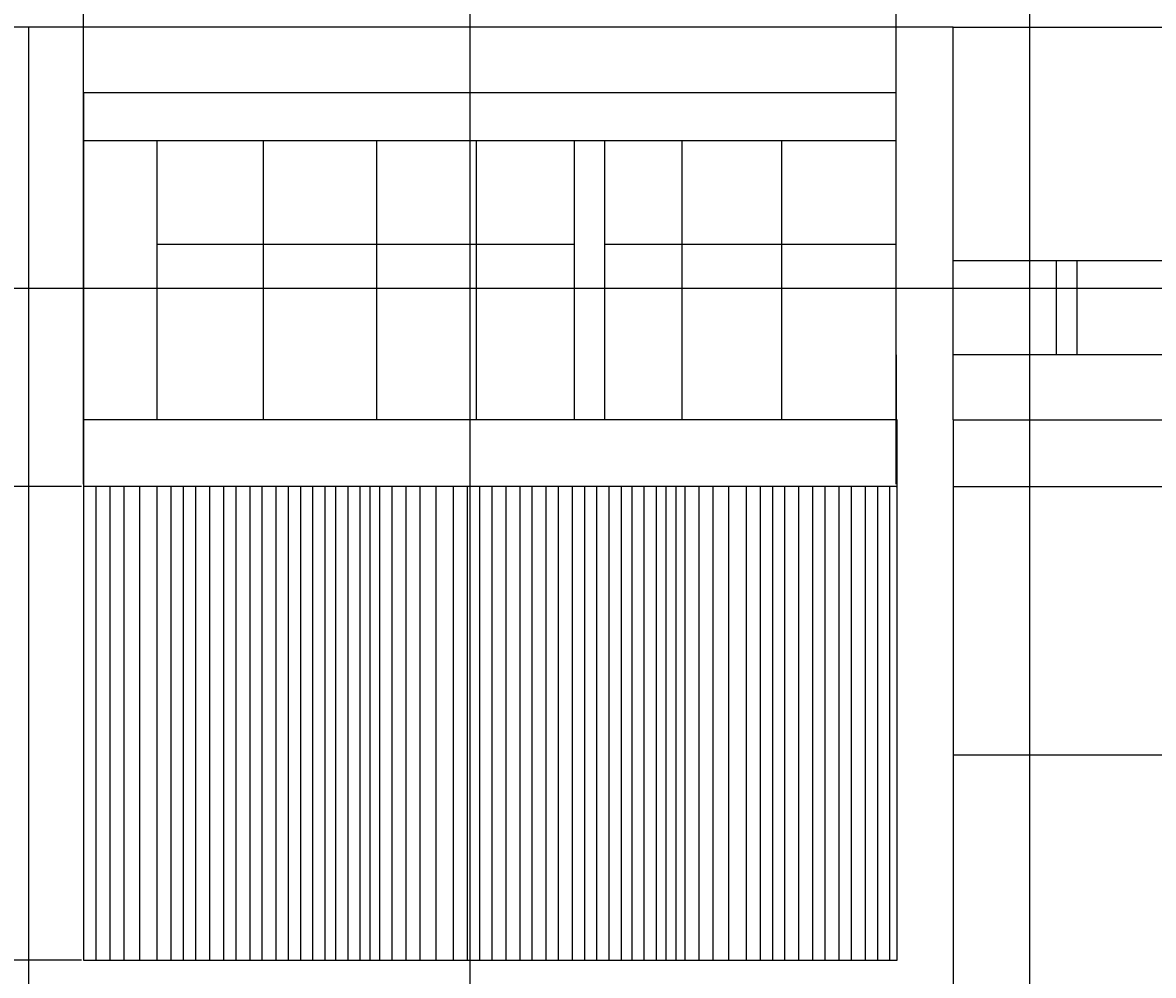
# Model space of a CAD drawing. Units: inches. Extents: x -117 to 121, y -77 to 40.
# Tile 20 of 45: x -6 to 28, y -60 to -32. Entities that reach past the tile are written whole.
import ezdxf

# ---------------------------------------------------------------- set-up
doc = ezdxf.new("R2010")
doc.units = ezdxf.units.IN
doc.header["$MEASUREMENT"] = 0
doc.layers.add('A-ANNO-DIMS', color=2, linetype='Continuous', lineweight=18)
doc.layers.add('A-ELEV', color=7, linetype='Continuous', lineweight=25)
doc.styles.get("Standard").update_dxf_attribs({"font": 'arial.ttf'})
doc.dimstyles.get("Standard").update_dxf_attribs({"dimtxt": 0.18, "dimasz": 0.18, "dimexe": 0.18, "dimexo": 0.0625, "dimgap": 0.09, "dimtad": 0, "dimtih": 1, "dimtoh": 1, "dimdec": 4, "dimzin": 0, "dimdsep": 46, "dimtxsty": 'Standard', "dimcen": 0.09, "dimadec": 0, "dimazin": 0, "dimtfac": 1, "dimtdec": 4, "dimtofl": 0, "dimtmove": 0, "dimatfit": 3, "dimfxl": 1, "dimtolj": 1, "dimtzin": 0, "dimarcsym": 0})

# ---------------------------------------------------------------- blocks, each defined once
blk = doc.blocks.new('*D13')
at = {"layer": 'A-ANNO-DIMS', "color": 0, "lineweight": -2, "transparency": 16777216}
for p, q in [((-2.663, 27.063), (-117.024, 27.063)), ((-116.844, 26.883), (-116.844, -16.974)), ((-116.844, -61.196), (-116.844, -17.338)), ((-106.096, -61.376), (-117.024, -61.376))]:
    blk.add_line(p, q, dxfattribs=at)
at = {"layer": 'A-ANNO-DIMS', "color": 0, "transparency": 16777216}
for points in [[(-116.874, 26.883), (-116.814, 26.883), (-116.844, 27.063)], [(-116.874, -61.196), (-116.814, -61.196), (-116.844, -61.376)]]:
    blk.add_solid(points, dxfattribs=at)
at = {"layer": 'Defpoints', "color": 0, "transparency": 16777216}
for p in [(-2.6, 27.063), (-116.844, -61.376), (-106.034, -61.376)]:
    blk.add_point(p, dxfattribs=at)
at = {"layer": 'A-ANNO-DIMS', "color": 0, "transparency": 16777216, "insert": (-116.844, -17.156), "char_height": 0.18, "attachment_point": 5}
blk.add_mtext('\\A1;88.44', dxfattribs=at)
blk = doc.blocks.new('*D32')
at = {"layer": 'A-ANNO-DIMS', "color": 0, "lineweight": -2, "transparency": 16777216}
for p, q in [((-3.85, -45.55), (-3.85, 38.61)), ((-3.67, 38.43), (7.757, 38.43)), ((20.113, 38.43), (8.686, 38.43)), ((20.293, -45.55), (20.293, 38.61))]:
    blk.add_line(p, q, dxfattribs=at)
at = {"layer": 'A-ANNO-DIMS', "color": 0, "transparency": 16777216}
for points in [[(-3.67, 38.46), (-3.67, 38.4), (-3.85, 38.43)], [(20.113, 38.46), (20.113, 38.4), (20.293, 38.43)]]:
    blk.add_solid(points, dxfattribs=at)
at = {"layer": 'Defpoints', "color": 0, "transparency": 16777216}
for p in [(20.293, 38.43), (-3.85, -45.613), (20.293, -45.613)]:
    blk.add_point(p, dxfattribs=at)
at = {"layer": 'A-ANNO-DIMS', "color": 0, "transparency": 16777216, "insert": (8.222, 38.43), "char_height": 0.18, "attachment_point": 5}
blk.add_mtext('\\A1;24.142', dxfattribs=at)
blk = doc.blocks.new('*D37')
at = {"layer": 'A-ANNO-DIMS', "color": 0, "lineweight": -2, "transparency": 16777216}
for p, q in [((-3.912, -45.613), (-117.024, -45.613)), ((-116.844, -45.793), (-116.844, -52.47)), ((-116.844, -59.512), (-116.844, -52.834)), ((-3.912, -59.692), (-117.024, -59.692))]:
    blk.add_line(p, q, dxfattribs=at)
at = {"layer": 'A-ANNO-DIMS', "color": 0, "transparency": 16777216}
for points in [[(-116.874, -45.793), (-116.814, -45.793), (-116.844, -45.613)], [(-116.874, -59.512), (-116.814, -59.512), (-116.844, -59.692)]]:
    blk.add_solid(points, dxfattribs=at)
at = {"layer": 'Defpoints', "color": 0, "transparency": 16777216}
for p in [(-116.844, -45.613), (-3.85, -45.613), (-3.85, -59.692)]:
    blk.add_point(p, dxfattribs=at)
at = {"layer": 'A-ANNO-DIMS', "color": 0, "transparency": 16777216, "insert": (-116.844, -52.652), "char_height": 0.18, "attachment_point": 5}
blk.add_mtext('\\A1;14.079', dxfattribs=at)
blk = doc.blocks.new('*D49')
at = {"layer": 'A-ANNO-DIMS', "color": 0, "lineweight": -2, "transparency": 16777216}
for p, q in [((-45.422, -23.501), (120.84, -23.501)), ((120.66, -23.681), (120.66, -31.426)), ((120.66, -39.536), (120.66, -31.79)), ((-45.471, -39.716), (120.84, -39.716))]:
    blk.add_line(p, q, dxfattribs=at)
at = {"layer": 'A-ANNO-DIMS', "color": 0, "transparency": 16777216}
for points in [[(120.63, -23.681), (120.69, -23.681), (120.66, -23.501)], [(120.63, -39.536), (120.69, -39.536), (120.66, -39.716)]]:
    blk.add_solid(points, dxfattribs=at)
at = {"layer": 'Defpoints', "color": 0, "transparency": 16777216}
for p in [(-45.485, -23.501), (120.66, -23.501), (-45.533, -39.716)]:
    blk.add_point(p, dxfattribs=at)
at = {"layer": 'A-ANNO-DIMS', "color": 0, "transparency": 16777216, "insert": (120.66, -31.608), "char_height": 0.18, "attachment_point": 5}
blk.add_mtext('\\A1;16.215', dxfattribs=at)
blk = doc.blocks.new('*D56')
at = {"layer": 'A-ANNO-DIMS', "color": 0, "lineweight": -2, "transparency": 16777216}
for p, q in [((-14.23, -7.853), (-14.23, -77.193)), ((7.628, -8.105), (7.628, -77.193)), ((-14.05, -77.013), (-3.766, -77.013)), ((7.448, -77.013), (-2.835, -77.013))]:
    blk.add_line(p, q, dxfattribs=at)
at = {"layer": 'A-ANNO-DIMS', "color": 0, "transparency": 16777216}
for points in [[(-14.05, -76.983), (-14.05, -77.043), (-14.23, -77.013)], [(7.448, -76.983), (7.448, -77.043), (7.628, -77.013)]]:
    blk.add_solid(points, dxfattribs=at)
at = {"layer": 'Defpoints', "color": 0, "transparency": 16777216}
for p in [(-14.23, -7.791), (7.628, -8.042), (7.628, -77.013)]:
    blk.add_point(p, dxfattribs=at)
at = {"layer": 'A-ANNO-DIMS', "color": 0, "transparency": 16777216, "insert": (-3.301, -77.013), "char_height": 0.18, "attachment_point": 5}
blk.add_mtext('\\A1;21.858', dxfattribs=at)
blk = doc.blocks.new('*D57')
at = {"layer": 'A-ANNO-DIMS', "color": 0, "lineweight": -2, "transparency": 16777216}
for p, q in [((7.628, -8.105), (7.628, -77.193)), ((24.248, -8.105), (24.248, -77.193)), ((7.808, -77.013), (15.483, -77.013)), ((24.068, -77.013), (16.393, -77.013))]:
    blk.add_line(p, q, dxfattribs=at)
at = {"layer": 'A-ANNO-DIMS', "color": 0, "transparency": 16777216}
for points in [[(7.808, -76.983), (7.808, -77.043), (7.628, -77.013)], [(24.068, -76.983), (24.068, -77.043), (24.248, -77.013)]]:
    blk.add_solid(points, dxfattribs=at)
at = {"layer": 'Defpoints', "color": 0, "transparency": 16777216}
for p in [(7.628, -8.042), (24.248, -8.042), (24.248, -77.013)]:
    blk.add_point(p, dxfattribs=at)
at = {"layer": 'A-ANNO-DIMS', "color": 0, "transparency": 16777216, "insert": (15.938, -77.013), "char_height": 0.18, "attachment_point": 5}
blk.add_mtext('\\A1;16.620', dxfattribs=at)
blk = doc.blocks.new('*D58')
at = {"layer": 'A-ANNO-DIMS', "color": 0, "lineweight": -2, "transparency": 16777216}
for p, q in [((57.61, -7.947), (57.61, -77.193)), ((24.248, -8.105), (24.248, -77.193)), ((24.428, -77.013), (40.467, -77.013)), ((57.43, -77.013), (41.392, -77.013))]:
    blk.add_line(p, q, dxfattribs=at)
at = {"layer": 'A-ANNO-DIMS', "color": 0, "transparency": 16777216}
for points in [[(24.428, -76.983), (24.428, -77.043), (24.248, -77.013)], [(57.43, -76.983), (57.43, -77.043), (57.61, -77.013)]]:
    blk.add_solid(points, dxfattribs=at)
at = {"layer": 'Defpoints', "color": 0, "transparency": 16777216}
for p in [(24.248, -8.042), (57.61, -7.885), (57.61, -77.013)]:
    blk.add_point(p, dxfattribs=at)
at = {"layer": 'A-ANNO-DIMS', "color": 0, "transparency": 16777216, "insert": (40.929, -77.013), "char_height": 0.18, "attachment_point": 5}
blk.add_mtext('\\A1;33.362', dxfattribs=at)

msp = doc.modelspace()

# ---------------------------------------------------------------- linework, layer by layer
at = {"layer": 'A-ELEV'}
for p, q in [((-5.4823, -31.9617), (-35.7647, -31.9617)), ((21.9795, -31.9617), (-5.4823, -31.9617)), ((-5.4823, -31.9617), (-5.4823, -61.3756)), ((21.9795, -43.6334), (21.9795, -31.9617)), ((21.9795, -31.9617), (38.5013, -31.9617)), ((20.2929, -33.9095), (-3.8495, -33.9095)), ((-3.8495, -33.9095), (-3.8495, -59.692)), ((20.2929, -41.7053), (20.2929, -33.9095)), ((-3.8495, -35.3307), (20.2929, -35.3307)), ((-1.662, -43.6334), (-1.662, -35.3307)), ((1.5002, -43.6334), (1.5002, -35.3307)), ((4.8599, -43.6334), (4.8599, -35.3307)), ((7.8276, -43.6334), (7.8276, -35.3307)), ((10.7393, -43.6334), (10.7393, -35.3307)), ((11.6413, -43.6334), (11.6413, -35.3307)), ((13.931, -43.6334), (13.931, -35.3307)), ((16.8987, -43.6334), (16.8987, -35.3307)), ((-1.662, -38.4117), (10.7393, -38.4117)), ((11.6413, -38.4117), (20.2929, -38.4117)), ((21.9795, -38.9022), (54.143, -38.9022)), ((25.0479, -41.7053), (25.0479, -38.9022)), ((25.6616, -41.7053), (25.6616, -38.9022)), ((20.2929, -41.7053), (20.2929, -43.6334)), ((37.6294, -41.7053), (21.9795, -41.7053)), ((20.3187, -43.6334), (-3.8495, -43.6334)), ((20.2929, -43.6334), (20.3187, -43.6334)), ((20.3187, -59.692), (20.3187, -43.6334)), ((21.9795, -43.6334), (21.9795, -61.3756)), ((21.9795, -43.6334), (57.4328, -43.6334)), ((20.3187, -45.6125), (-3.8495, -45.6125)), ((-3.4755, -59.692), (-3.4755, -45.6125)), ((-3.0598, -59.692), (-3.0598, -45.6125)), ((-2.6441, -59.692), (-2.6441, -45.6125)), ((-2.1764, -59.692), (-2.1764, -45.6125)), ((-1.6568, -59.692), (-1.6568, -45.6125)), ((-1.2411, -59.692), (-1.2411, -45.6125)), ((-0.8773, -59.692), (-0.8773, -45.6125)), ((-0.5136, -59.692), (-0.5136, -45.6125)), ((-0.0979, -59.692), (-0.0979, -45.6125)), ((0.3178, -59.692), (0.3178, -45.6125)), ((0.6816, -59.692), (0.6816, -45.6125)), ((1.0973, -59.692), (1.0973, -45.6125)), ((1.461, -59.692), (1.461, -45.6125)), ((1.8767, -59.692), (1.8767, -45.6125)), ((2.2405, -59.692), (2.2405, -45.6125)), ((2.6042, -59.692), (2.6042, -45.6125)), ((2.968, -59.692), (2.968, -45.6125)), ((3.3317, -59.692), (3.3317, -45.6125)), ((3.6515, -59.692), (3.6515, -45.6125)), ((4.01, -59.692), (4.01, -45.6125)), ((4.3685, -59.692), (4.3685, -45.6125)), ((4.6618, -59.692), (4.6618, -45.6125)), ((4.9551, -59.692), (4.9551, -45.6125)), ((5.324, -59.692), (5.324, -45.6125)), ((5.7397, -59.692), (5.7397, -45.6125)), ((6.1554, -59.692), (6.1554, -45.6125)), ((6.623, -59.692), (6.623, -45.6125)), ((7.1427, -59.692), (7.1427, -45.6125)), ((7.5584, -59.692), (7.5584, -45.6125)), ((7.9221, -59.692), (7.9221, -45.6125)), ((8.2859, -59.692), (8.2859, -45.6125)), ((8.7016, -59.692), (8.7016, -45.6125)), ((9.1173, -59.692), (9.1173, -45.6125)), ((9.481, -59.692), (9.481, -45.6125)), ((9.8967, -59.692), (9.8967, -45.6125)), ((10.2605, -59.692), (10.2605, -45.6125)), ((10.6762, -59.692), (10.6762, -45.6125)), ((11.0399, -59.692), (11.0399, -45.6125)), ((11.4037, -59.692), (11.4037, -45.6125)), ((11.7674, -59.692), (11.7674, -45.6125)), ((12.1311, -59.692), (12.1311, -45.6125)), ((12.4509, -59.692), (12.4509, -45.6125)), ((12.8094, -59.692), (12.8094, -45.6125)), ((13.1679, -59.692), (13.1679, -45.6125)), ((13.4612, -59.692), (13.4612, -45.6125)), ((13.7546, -59.692), (13.7546, -45.6125)), ((14.0256, -59.692), (14.0256, -45.6125)), ((14.4413, -59.692), (14.4413, -45.6125)), ((14.857, -59.692), (14.857, -45.6125)), ((15.3247, -59.692), (15.3247, -45.6125)), ((15.8443, -59.692), (15.8443, -45.6125)), ((16.26, -59.692), (16.26, -45.6125)), ((16.6238, -59.692), (16.6238, -45.6125)), ((16.9875, -59.692), (16.9875, -45.6125)), ((17.4032, -59.692), (17.4032, -45.6125)), ((17.8189, -59.692), (17.8189, -45.6125)), ((18.1827, -59.692), (18.1827, -45.6125)), ((18.5984, -59.692), (18.5984, -45.6125)), ((18.9621, -59.692), (18.9621, -45.6125)), ((19.3778, -59.692), (19.3778, -45.6125)), ((19.7416, -59.692), (19.7416, -45.6125)), ((20.1053, -59.692), (20.1053, -45.6125)), ((20.2929, -45.6125), (20.3187, -45.6125)), ((21.9795, -45.6125), (37.9123, -45.6125)), ((21.9795, -53.5899), (37.9123, -53.5899)), ((-3.8495, -59.692), (20.3187, -59.692))]:
    msp.add_line(p, q, dxfattribs=at)

# ---------------------------------------------------------------- dimensions: what is measured, and where the dimension line sits
at = {"layer": 'A-ANNO-DIMS'}
for base, p1, p2, picture, middle in [((20.2929, 38.4297), (-3.8495, -45.6125), (20.2929, -45.6125), '*D32', (8.2217, 38.4297)), ((7.6284, -77.0135), (-14.2298, -7.7907), (7.6284, -8.0421), '*D56', (-3.3007, -77.0135)), ((24.2481, -77.0135), (7.6284, -8.0421), (24.2481, -8.0421), '*D57', (15.9383, -77.0135)), ((57.6104, -77.0135), (24.2481, -8.0421), (57.6104, -7.8846), '*D58', (40.9293, -77.0135))]:
    dim = msp.add_linear_dim(base=base, p1=p1, p2=p2, dimstyle='Standard', override={"dimdec": 3, "dimlfac": 1, "dimrnd": 0, "dimzin": 0, "dimdsep": 46, "dimlunit": 2}, dxfattribs=at)
    dim.commit()
    dim.dimension.update_dxf_attribs({"geometry": picture, "text_midpoint": middle})
for base, p1, p2, override, picture, middle in [((-116.8438, -61.3756), (-2.6001, 27.0634), (-106.0338, -61.3756), {"dimdec": 2, "dimlfac": 1, "dimrnd": 0, "dimzin": 0, "dimdsep": 46, "dimlunit": 2}, '*D13', (-116.8438, -17.1561)), ((120.6602, -23.5007), (-45.5331, -39.716), (-45.4848, -23.5007), {"dimdec": 3, "dimlfac": 1, "dimrnd": 0, "dimzin": 0, "dimdsep": 46, "dimlunit": 2}, '*D49', (120.6602, -31.6083)), ((-116.843772, -45.612514), (-3.849514, -59.692012), (-3.849514, -45.612514), {"dimdec": 3, "dimlfac": 1, "dimrnd": 0, "dimzin": 0, "dimdsep": 46, "dimlunit": 2}, '*D37', (-116.843772, -52.652263))]:
    dim = msp.add_linear_dim(base=base, p1=p1, p2=p2, angle=90, dimstyle='Standard', override=override, dxfattribs=at)
    dim.commit()
    dim.dimension.update_dxf_attribs({"geometry": picture, "text_midpoint": middle})

doc.saveas('drawing.dxf')
